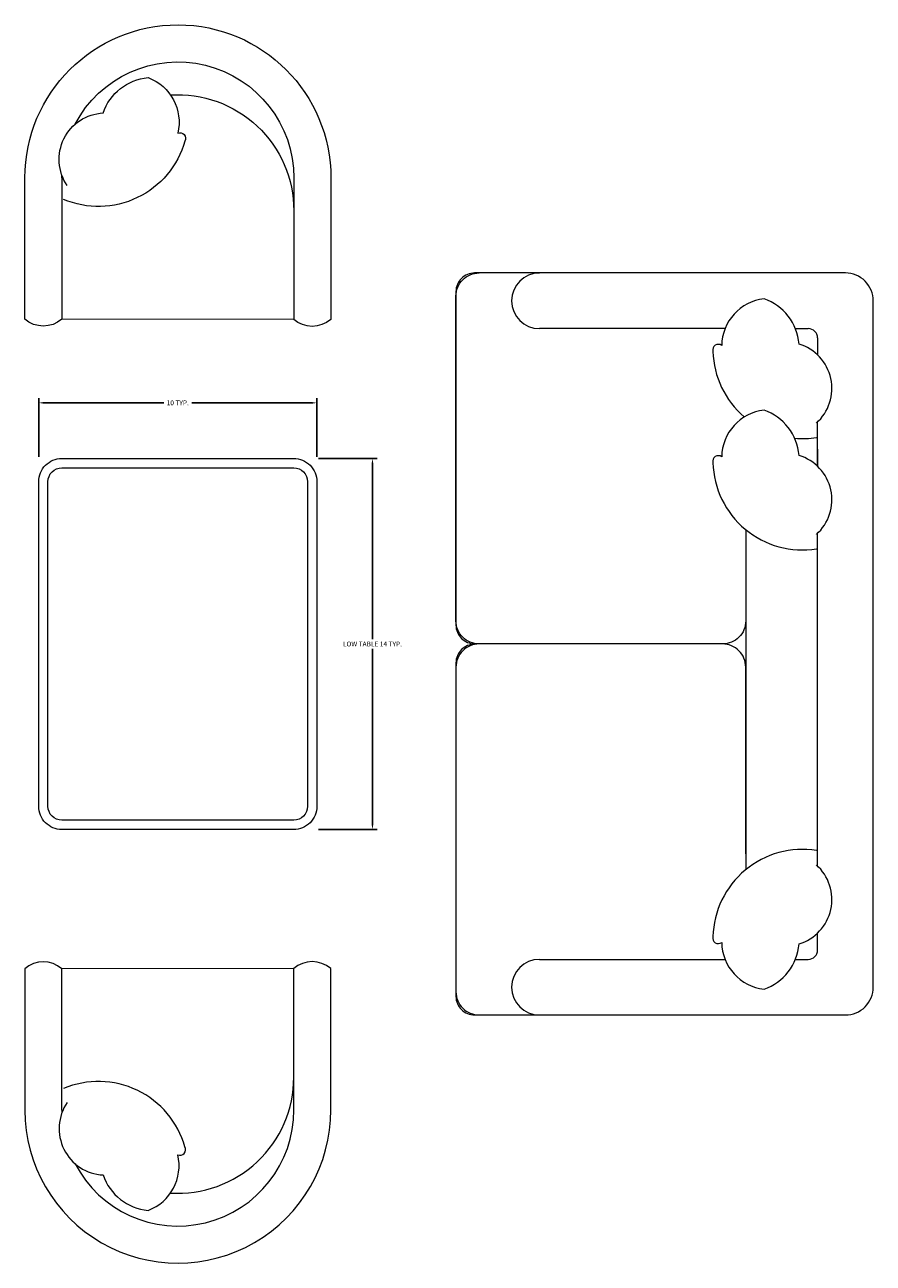
# Model space of a CAD drawing. Units: inches. Extents: x 1885 to 2748, y 783 to 2421.
# Tile 106 of 117: x 2453 to 2485, y 1980 to 2026. Entities that reach past the tile are written whole.
import ezdxf

# ---------------------------------------------------------------- set-up
doc = ezdxf.new("R2010")
doc.units = ezdxf.units.IN
doc.layers.add('A-ANNO-DIMS', color=2, linetype='Continuous', lineweight=18)
doc.layers.add('A-FURN', color=8, linetype='Continuous', lineweight=13)
doc.styles.get("Standard").update_dxf_attribs({"font": 'arial.ttf'})
doc.dimstyles.get("Standard").update_dxf_attribs({"dimtxt": 0.18, "dimasz": 0.18, "dimexe": 0.18, "dimexo": 0.0625, "dimgap": 0.09, "dimtad": 0, "dimtih": 1, "dimtoh": 1, "dimdec": 4, "dimzin": 0, "dimdsep": 46, "dimtxsty": 'Standard', "dimcen": 0.09, "dimadec": 0, "dimazin": 0, "dimtfac": 1, "dimtdec": 4, "dimtofl": 0, "dimtmove": 0, "dimatfit": 3, "dimfxl": 1, "dimtolj": 1, "dimtzin": 0, "dimarcsym": 0})

# ---------------------------------------------------------------- blocks, each defined once
blk = doc.blocks.new('A$C1352')
at = {"color": 0}
for points in [[(0.0027, 0.053), (0.0027, 0.553, -0.414214), (0.0527, 0.603), (0.7527, 0.603, -0.414214), (0.8027, 0.553), (0.8027, 0.053, -0.414214), (0.7527, 0.003), (0.0527, 0.003, -0.414214)], [(0.0227, 0.053), (0.0227, 0.553, -0.414214), (0.0527, 0.583), (0.7527, 0.583, -0.414214), (0.7827, 0.553), (0.7827, 0.053, -0.414214), (0.7527, 0.023), (0.0527, 0.023, -0.414214)]]:
    blk.add_lwpolyline(points, format="xyb", close=True, dxfattribs=at)
blk = doc.blocks.new('CHAIR-LOUNGE')
blk.add_line((1.388, 5.701), (1.383, 10.98))
at = {"ltscale": 0.03}
blk.add_lwpolyline([(1.383, 10.98, 0.369229), (-0.002, 10.979), (0.003, 5.7, 1), (11.423, 5.711), (11.418, 10.99, 0.369229), (10.034, 10.988)], format="xyb", close=True, dxfattribs=at)
blk.add_lwpolyline([(1.877, 3.707, 0.785087), (10.039, 5.71), (10.034, 10.988)], format="xyb")
for centre, radius, start, end in [((5.712, 6.928), 4.326, 266.342, 0.0539), ((2.748, 3.424), 3.35, 15.7143, 112.9857), ((3.014, 5.016), 1.734, 145.8599, 267.0078), ((5.713, 5.706), 4.326, 180.0539, 181.1464), ((5.792, 4.23), 0.207, 246.2577, 29.3762), ((3.979, 3.63), 1.778, 290.5305, 13.3597), ((4.772, 3.909), 1.951, 198.6466, 265.0001)]:
    blk.add_arc(centre, radius, start, end)
blk = doc.blocks.new('*D31')
at = {"layer": 'A-ANNO-DIMS', "color": 0, "lineweight": -2, "transparency": 16777216}
for p, q in [((2463.97, 2010.149), (2466.163, 2010.149)), ((2465.983, 2009.969), (2465.983, 2003.411)), ((2465.983, 1996.487), (2465.983, 2003.044)), ((2463.97, 1996.307), (2466.163, 1996.307))]:
    blk.add_line(p, q, dxfattribs=at)
at = {"layer": 'A-ANNO-DIMS', "color": 0, "transparency": 16777216}
for points in [[(2465.953, 2009.969), (2466.013, 2009.969), (2465.983, 2010.149)], [(2465.953, 1996.487), (2466.013, 1996.487), (2465.983, 1996.307)]]:
    blk.add_solid(points, dxfattribs=at)
at = {"layer": 'Defpoints', "color": 0, "transparency": 16777216}
for p in [(2463.907, 2010.149), (2463.907, 1996.307), (2465.983, 1996.307)]:
    blk.add_point(p, dxfattribs=at)
at = {"layer": 'A-ANNO-DIMS', "color": 0, "transparency": 16777216, "insert": (2465.983, 2003.228), "char_height": 0.18, "attachment_point": 5}
blk.add_mtext('\\A1;LOW TABLE 14 TYP.', dxfattribs=at)
blk = doc.blocks.new('*D32')
at = {"layer": 'A-ANNO-DIMS', "color": 0, "lineweight": -2, "transparency": 16777216}
for p, q in [((2453.526, 2010.211), (2453.526, 2012.405)), ((2463.907, 2010.211), (2463.907, 2012.405)), ((2453.706, 2012.225), (2458.197, 2012.225)), ((2463.727, 2012.225), (2459.236, 2012.225))]:
    blk.add_line(p, q, dxfattribs=at)
at = {"layer": 'A-ANNO-DIMS', "color": 0, "transparency": 16777216}
for points in [[(2453.706, 2012.255), (2453.706, 2012.195), (2453.526, 2012.225)], [(2463.727, 2012.255), (2463.727, 2012.195), (2463.907, 2012.225)]]:
    blk.add_solid(points, dxfattribs=at)
at = {"layer": 'Defpoints', "color": 0, "transparency": 16777216}
for p in [(2463.907, 2012.225), (2453.526, 2010.149), (2463.907, 2010.149)]:
    blk.add_point(p, dxfattribs=at)
at = {"layer": 'A-ANNO-DIMS', "color": 0, "transparency": 16777216, "insert": (2458.716, 2012.225), "char_height": 0.18, "attachment_point": 5}
blk.add_mtext('\\A1;10 TYP.', dxfattribs=at)

msp = doc.modelspace()

# ---------------------------------------------------------------- linework, layer by layer
at = {"layer": 'A-FURN'}
for p, q in [((2479.139, 2014.993), (2472.212, 2014.993)), ((2481.766, 2014.993), (2482.248, 2014.993)), ((2482.594, 2014.647), (2482.594, 2014.011)), ((2482.594, 2009.856), (2482.594, 2011.512)), ((2482.594, 2010.493), (2482.594, 2009.856)), ((2482.594, 1994.943), (2482.594, 2007.358)), ((2482.594, 1991.808), (2482.594, 1992.445)), ((2472.212, 1991.462), (2479.139, 1991.462)), ((2481.766, 1991.462), (2482.248, 1991.462))]:
    msp.add_line(p, q, dxfattribs=at)
at = {"layer": 'A-FURN', "ltscale": 0.03}
msp.add_lwpolyline([(2469.79, 2003.219, 0.414214), (2469.098, 2002.527), (2469.098, 1990.078, 0.414214), (2469.79, 1989.386), (2483.632, 1989.386, 0.414214), (2484.67, 1990.424), (2484.67, 2016.031, 0.414214), (2483.632, 2017.07), (2469.79, 2017.07, 0.414214), (2469.098, 2016.378), (2469.098, 2003.928, 0.414214), (2469.79, 2003.236)], format="xyb", dxfattribs=at)
at = {"layer": 'A-FURN'}
for points in [[(2479.912, 2007.497), (2479.912, 2004.093, -0.414214), (2479.047, 2003.228), (2469.963, 2003.228, -0.414214), (2469.098, 2004.093), (2469.098, 2016.204, -0.414214), (2469.963, 2017.07)], [(2479.912, 1995.393), (2479.912, 2002.362, 0.414214), (2479.047, 2003.228), (2469.963, 2003.228, 0.414214), (2469.098, 2002.362), (2469.098, 1990.251, 0.414214), (2469.963, 1989.386)]]:
    msp.add_lwpolyline(points, format="xyb", dxfattribs=at)
msp.add_lwpolyline([(2479.912, 2007.497), (2479.912, 1994.804)], dxfattribs=at)
for centre, radius, start, end in [((2472.212, 2016.031), 1.038, 90, 180), ((2472.212, 2016.031), 1.038, 180, 270), ((2480.794, 2014.341), 1.778, 96.4279, 179.257), ((2479.956, 2014.264), 1.951, 4.5439, 70.8974), ((2482.248, 2014.647), 0.346, 0, 90), ((2482.248, 2014.647), 0.346, 0, 90), ((2478.889, 2014.201), 0.207, 52.155, 195.2735), ((2482.037, 2014.24), 3.35, 181.6116, 229.376), ((2481.392, 2012.762), 1.734, 311.7572, 72.9051), ((2480.794, 2010.187), 1.778, 96.4279, 179.257), ((2479.956, 2010.11), 1.951, 4.5439, 70.8974), ((2482.037, 2014.24), 3.35, 264.881, 278.883), ((2478.889, 2010.047), 0.207, 52.155, 195.2735), ((2482.037, 2010.086), 3.35, 181.6116, 278.883), ((2481.392, 2008.607), 1.734, 311.7572, 72.9051), ((2482.037, 1992.215), 3.35, 81.117, 178.3884), ((2481.392, 1993.694), 1.734, 287.0949, 48.2428), ((2478.889, 1992.255), 0.207, 164.7265, 307.845), ((2480.794, 1992.114), 1.778, 180.743, 263.5721), ((2479.956, 1992.191), 1.951, 289.1026, 355.4561), ((2482.248, 1991.808), 0.346, 270, 0), ((2472.212, 1990.424), 1.038, 90, 180), ((2472.212, 1990.424), 1.038, 180, 270)]:
    msp.add_arc(centre, radius, start, end, dxfattribs=at)

# ---------------------------------------------------------------- block references
at = {"layer": 'A-FURN', "extrusion": (0, 0, -1), "zscale": -1, "rotation": 180}
msp.add_blockref('CHAIR-LOUNGE', (-2453.008, 2026.324), dxfattribs=at)
at = {"layer": 'A-FURN', "ltscale": 0.03, "xscale": 17.30251319894821, "yscale": 17.30251319894821, "zscale": 17.30251319894821, "rotation": 270}
msp.add_blockref('A$C1352', (2453.474, 2010.195), dxfattribs=at)
at = {"layer": 'A-FURN'}
msp.add_blockref('CHAIR-LOUNGE', (2453.008, 1980.132), dxfattribs=at)

# ---------------------------------------------------------------- dimensions: what is measured, and where the dimension line sits
at = {"layer": 'A-ANNO-DIMS'}
dim = msp.add_linear_dim(base=(2463.907, 2012.225), p1=(2453.526, 2010.149), p2=(2463.907, 2010.149), text='<> TYP.', dimstyle='Standard', override={"dimdec": 0, "dimlfac": 1, "dimrnd": 0, "dimzin": 0, "dimdsep": 46, "dimlunit": 2}, dxfattribs=at)
dim.commit()
dim.dimension.update_dxf_attribs({"geometry": '*D32', "text_midpoint": (2458.716, 2012.225)})
dim = msp.add_linear_dim(base=(2465.983, 1996.307), p1=(2463.907, 2010.149), p2=(2463.907, 1996.307), angle=270, text='LOW TABLE <> TYP.', dimstyle='Standard', override={"dimdec": 0, "dimlfac": 1, "dimrnd": 0, "dimzin": 0, "dimdsep": 46, "dimlunit": 2}, dxfattribs=at)
dim.commit()
dim.dimension.update_dxf_attribs({"geometry": '*D31', "text_midpoint": (2465.983, 2003.228)})

doc.saveas('drawing.dxf')
